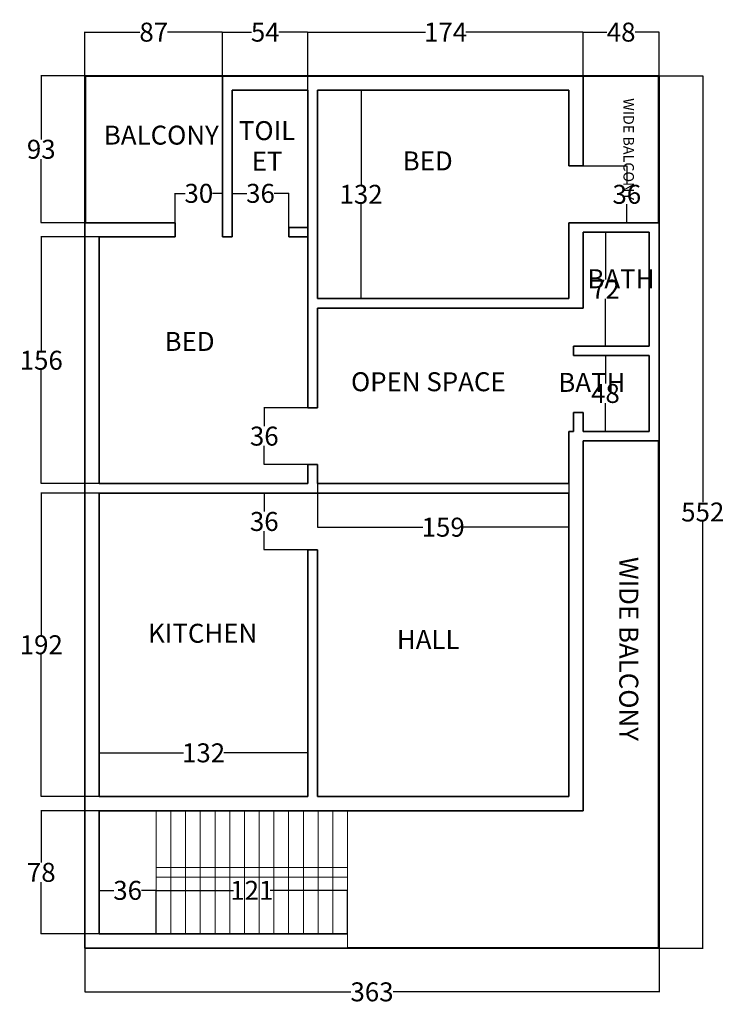
# Model space of a CAD drawing. Units: inches. Extents: x -24 to 1692, y -109 to 592.
# Tile 1 of 4: x -24 to 422, y -31 to 592. Entities that reach past the tile are written whole.
import ezdxf
from ezdxf.enums import TextEntityAlignment as Align

# ---------------------------------------------------------------- set-up
doc = ezdxf.new("R2010")
doc.units = ezdxf.units.IN
doc.header["$MEASUREMENT"] = 0
for name, color, linetype, lineweight in [('A-ANNO-DIMS', 2, 'Continuous', 18), ('A-AREA-IDEN', 7, 'Continuous', 18), ('A-FLOR-STRS', 2, 'Continuous', 18), ('A-WALL', 7, 'Continuous', 35)]:
    doc.layers.add(name, color=color, linetype=linetype, lineweight=lineweight)
doc.styles.get("Standard").update_dxf_attribs({"font": 'arial.ttf'})
doc.dimstyles.get("Standard").update_dxf_attribs({"dimtxt": 12, "dimasz": 0.18, "dimexe": 0.18, "dimexo": 0.0625, "dimgap": 0.09, "dimtad": 0, "dimtih": 1, "dimtoh": 1, "dimdec": 0, "dimzin": 0, "dimdsep": 46, "dimlunit": 4, "dimtxsty": 'Standard', "dimcen": 0.09, "dimadec": 0, "dimazin": 0, "dimtfac": 1, "dimtdec": 0, "dimtofl": 0, "dimtmove": 0, "dimatfit": 3, "dimfxl": 1, "dimtolj": 1, "dimtzin": 0, "dimarcsym": 0})

# ---------------------------------------------------------------- blocks, each defined once
blk = doc.blocks.new('*D11')
at = {"layer": 'A-ANNO-DIMS', "color": 0, "lineweight": -2, "transparency": 16777216}
for p, q in [((17.56, 4), (17.56, -23.73)), ((380.56, 4), (380.56, -23.73)), ((17.74, -23.55), (185.71, -23.55)), ((380.38, -23.55), (212.4, -23.55))]:
    blk.add_line(p, q, dxfattribs=at)
at = {"layer": 'A-ANNO-DIMS', "color": 0, "transparency": 16777216}
for points in [[(17.74, -23.52), (17.74, -23.58), (17.56, -23.55)], [(380.38, -23.52), (380.38, -23.58), (380.56, -23.55)]]:
    blk.add_solid(points, dxfattribs=at)
at = {"layer": 'Defpoints', "color": 0, "transparency": 16777216}
for p in [(17.56, 4.07), (380.56, 4.07), (380.56, -23.55)]:
    blk.add_point(p, dxfattribs=at)
at = {"layer": 'A-ANNO-DIMS', "color": 0, "transparency": 16777216, "insert": (199.06, -23.55), "char_height": 12, "attachment_point": 5}
blk.add_mtext('\\A1;363', dxfattribs=at)
blk = doc.blocks.new('*D12')
at = {"layer": 'A-ANNO-DIMS', "color": 0, "lineweight": -2, "transparency": 16777216}
for p, q in [((380.62, 556.07), (408.35, 556.07)), ((408.17, 555.89), (408.17, 286.28)), ((408.17, 4.25), (408.17, 273.85)), ((380.62, 4.07), (408.35, 4.07))]:
    blk.add_line(p, q, dxfattribs=at)
at = {"layer": 'A-ANNO-DIMS', "color": 0, "transparency": 16777216}
for points in [[(408.14, 555.89), (408.2, 555.89), (408.17, 556.07)], [(408.14, 4.25), (408.2, 4.25), (408.17, 4.07)]]:
    blk.add_solid(points, dxfattribs=at)
at = {"layer": 'Defpoints', "color": 0, "transparency": 16777216}
for p in [(380.56, 556.07), (408.17, 556.07), (380.56, 4.07)]:
    blk.add_point(p, dxfattribs=at)
at = {"layer": 'A-ANNO-DIMS', "color": 0, "transparency": 16777216, "insert": (408.17, 280.07), "char_height": 12, "attachment_point": 5}
blk.add_mtext('\\A1;552', dxfattribs=at)
blk = doc.blocks.new('*D13')
at = {"layer": 'A-ANNO-DIMS', "color": 0, "lineweight": -2, "transparency": 16777216}
for p, q in [((17.56, 556.13), (17.56, 583.86)), ((17.74, 583.68), (52.36, 583.68)), ((104.38, 583.68), (69.75, 583.68)), ((104.56, 555.83), (104.56, 583.86))]:
    blk.add_line(p, q, dxfattribs=at)
at = {"layer": 'A-ANNO-DIMS', "color": 0, "transparency": 16777216}
for points in [[(17.74, 583.71), (17.74, 583.65), (17.56, 583.68)], [(104.38, 583.71), (104.38, 583.65), (104.56, 583.68)]]:
    blk.add_solid(points, dxfattribs=at)
at = {"layer": 'Defpoints', "color": 0, "transparency": 16777216}
for p in [(104.56, 583.68), (17.56, 556.07), (104.56, 555.77)]:
    blk.add_point(p, dxfattribs=at)
at = {"layer": 'A-ANNO-DIMS', "color": 0, "transparency": 16777216, "insert": (61.06, 583.68), "char_height": 12, "attachment_point": 5}
blk.add_mtext('\\A1;87', dxfattribs=at)
blk = doc.blocks.new('*D14')
at = {"layer": 'A-ANNO-DIMS', "color": 0, "lineweight": -2, "transparency": 16777216}
for p, q in [((104.56, 555.83), (104.56, 583.86)), ((104.74, 583.68), (122.9, 583.68)), ((158.38, 583.68), (140.22, 583.68)), ((158.56, 547.13), (158.56, 583.86))]:
    blk.add_line(p, q, dxfattribs=at)
at = {"layer": 'A-ANNO-DIMS', "color": 0, "transparency": 16777216}
for points in [[(104.74, 583.71), (104.74, 583.65), (104.56, 583.68)], [(158.38, 583.71), (158.38, 583.65), (158.56, 583.68)]]:
    blk.add_solid(points, dxfattribs=at)
at = {"layer": 'Defpoints', "color": 0, "transparency": 16777216}
for p in [(158.56, 583.68), (104.56, 555.77), (158.56, 547.07)]:
    blk.add_point(p, dxfattribs=at)
at = {"layer": 'A-ANNO-DIMS', "color": 0, "transparency": 16777216, "insert": (131.56, 583.68), "char_height": 12, "attachment_point": 5}
blk.add_mtext('\\A1;54', dxfattribs=at)
blk = doc.blocks.new('*D15')
at = {"layer": 'A-ANNO-DIMS', "color": 0, "lineweight": -2, "transparency": 16777216}
for p, q in [((158.56, 547.13), (158.56, 583.86)), ((158.74, 583.68), (232.8, 583.68)), ((332.38, 583.68), (258.31, 583.68)), ((332.56, 556.13), (332.56, 583.86))]:
    blk.add_line(p, q, dxfattribs=at)
at = {"layer": 'A-ANNO-DIMS', "color": 0, "transparency": 16777216}
for points in [[(158.74, 583.71), (158.74, 583.65), (158.56, 583.68)], [(332.38, 583.71), (332.38, 583.65), (332.56, 583.68)]]:
    blk.add_solid(points, dxfattribs=at)
at = {"layer": 'Defpoints', "color": 0, "transparency": 16777216}
for p in [(332.56, 583.68), (332.56, 556.07), (158.56, 547.07)]:
    blk.add_point(p, dxfattribs=at)
at = {"layer": 'A-ANNO-DIMS', "color": 0, "transparency": 16777216, "insert": (245.56, 583.68), "char_height": 12, "attachment_point": 5}
blk.add_mtext('\\A1;174', dxfattribs=at)
blk = doc.blocks.new('*D16')
at = {"layer": 'A-ANNO-DIMS', "color": 0, "lineweight": -2, "transparency": 16777216}
for p, q in [((332.56, 556.13), (332.56, 583.86)), ((332.74, 583.68), (347.62, 583.68)), ((380.38, 583.68), (365.49, 583.68)), ((380.56, 556.13), (380.56, 583.86))]:
    blk.add_line(p, q, dxfattribs=at)
at = {"layer": 'A-ANNO-DIMS', "color": 0, "transparency": 16777216}
for points in [[(332.74, 583.71), (332.74, 583.65), (332.56, 583.68)], [(380.38, 583.71), (380.38, 583.65), (380.56, 583.68)]]:
    blk.add_solid(points, dxfattribs=at)
at = {"layer": 'Defpoints', "color": 0, "transparency": 16777216}
for p in [(380.56, 583.68), (332.56, 556.07), (380.56, 556.07)]:
    blk.add_point(p, dxfattribs=at)
at = {"layer": 'A-ANNO-DIMS', "color": 0, "transparency": 16777216, "insert": (356.56, 583.68), "char_height": 12, "attachment_point": 5}
blk.add_mtext('\\A1;48', dxfattribs=at)
blk = doc.blocks.new('*D17')
at = {"layer": 'A-ANNO-DIMS', "color": 0, "lineweight": -2, "transparency": 16777216}
for p, q in [((26.49, 91.07), (-10.24, 91.07)), ((-10.06, 90.89), (-10.06, 58.28)), ((-10.06, 13.25), (-10.06, 45.85)), ((26.49, 13.07), (-10.24, 13.07))]:
    blk.add_line(p, q, dxfattribs=at)
at = {"layer": 'A-ANNO-DIMS', "color": 0, "transparency": 16777216}
for points in [[(-10.09, 90.89), (-10.03, 90.89), (-10.06, 91.07)], [(-10.09, 13.25), (-10.03, 13.25), (-10.06, 13.07)]]:
    blk.add_solid(points, dxfattribs=at)
at = {"layer": 'Defpoints', "color": 0, "transparency": 16777216}
for p in [(-10.06, 91.07), (26.56, 91.07), (26.56, 13.07)]:
    blk.add_point(p, dxfattribs=at)
at = {"layer": 'A-ANNO-DIMS', "color": 0, "transparency": 16777216, "insert": (-10.06, 52.07), "char_height": 12, "attachment_point": 5}
blk.add_mtext('\\A1;78', dxfattribs=at)
blk = doc.blocks.new('*D18')
at = {"layer": 'A-ANNO-DIMS', "color": 0, "lineweight": -2, "transparency": 16777216}
for p, q in [((26.49, 292.07), (-10.24, 292.07)), ((-10.06, 291.89), (-10.06, 202.28)), ((-10.06, 100.25), (-10.06, 189.85)), ((26.49, 100.07), (-10.24, 100.07))]:
    blk.add_line(p, q, dxfattribs=at)
at = {"layer": 'A-ANNO-DIMS', "color": 0, "transparency": 16777216}
for points in [[(-10.09, 291.89), (-10.03, 291.89), (-10.06, 292.07)], [(-10.09, 100.25), (-10.03, 100.25), (-10.06, 100.07)]]:
    blk.add_solid(points, dxfattribs=at)
at = {"layer": 'Defpoints', "color": 0, "transparency": 16777216}
for p in [(-10.06, 292.07), (26.56, 292.07), (26.56, 100.07)]:
    blk.add_point(p, dxfattribs=at)
at = {"layer": 'A-ANNO-DIMS', "color": 0, "transparency": 16777216, "insert": (-10.06, 196.07), "char_height": 12, "attachment_point": 5}
blk.add_mtext('\\A1;192', dxfattribs=at)
blk = doc.blocks.new('*D19')
at = {"layer": 'A-ANNO-DIMS', "color": 0, "lineweight": -2, "transparency": 16777216}
for p, q in [((26.49, 454.07), (-10.24, 454.07)), ((-10.06, 453.89), (-10.06, 382.28)), ((-10.06, 298.25), (-10.06, 369.85)), ((26.49, 298.07), (-10.24, 298.07))]:
    blk.add_line(p, q, dxfattribs=at)
at = {"layer": 'A-ANNO-DIMS', "color": 0, "transparency": 16777216}
for points in [[(-10.09, 453.89), (-10.03, 453.89), (-10.06, 454.07)], [(-10.09, 298.25), (-10.03, 298.25), (-10.06, 298.07)]]:
    blk.add_solid(points, dxfattribs=at)
at = {"layer": 'Defpoints', "color": 0, "transparency": 16777216}
for p in [(-10.06, 454.07), (26.56, 454.07), (26.56, 298.07)]:
    blk.add_point(p, dxfattribs=at)
at = {"layer": 'A-ANNO-DIMS', "color": 0, "transparency": 16777216, "insert": (-10.06, 376.07), "char_height": 12, "attachment_point": 5}
blk.add_mtext('\\A1;156', dxfattribs=at)
blk = doc.blocks.new('*D20')
at = {"layer": 'A-ANNO-DIMS', "color": 0, "lineweight": -2, "transparency": 16777216}
for p, q in [((17.49, 556.07), (-10.24, 556.07)), ((-10.06, 555.89), (-10.06, 515.79)), ((-10.06, 463.25), (-10.06, 503.34)), ((17.49, 463.07), (-10.24, 463.07))]:
    blk.add_line(p, q, dxfattribs=at)
at = {"layer": 'A-ANNO-DIMS', "color": 0, "transparency": 16777216}
for points in [[(-10.09, 555.89), (-10.03, 555.89), (-10.06, 556.07)], [(-10.09, 463.25), (-10.03, 463.25), (-10.06, 463.07)]]:
    blk.add_solid(points, dxfattribs=at)
at = {"layer": 'Defpoints', "color": 0, "transparency": 16777216}
for p in [(-10.06, 556.07), (17.56, 556.07), (17.56, 463.07)]:
    blk.add_point(p, dxfattribs=at)
at = {"layer": 'A-ANNO-DIMS', "color": 0, "transparency": 16777216, "insert": (-10.06, 509.57), "char_height": 12, "attachment_point": 5}
blk.add_mtext('\\A1;93', dxfattribs=at)
blk = doc.blocks.new('*D21')
at = {"layer": 'A-ANNO-DIMS', "color": 0, "lineweight": -2, "transparency": 16777216}
for p, q in [((164.62, 547.07), (192.35, 547.07)), ((192.17, 546.89), (192.17, 487.29)), ((192.17, 415.25), (192.17, 474.84)), ((164.62, 415.07), (192.35, 415.07))]:
    blk.add_line(p, q, dxfattribs=at)
at = {"layer": 'A-ANNO-DIMS', "color": 0, "transparency": 16777216}
for points in [[(192.14, 546.89), (192.2, 546.89), (192.17, 547.07)], [(192.14, 415.25), (192.2, 415.25), (192.17, 415.07)]]:
    blk.add_solid(points, dxfattribs=at)
at = {"layer": 'Defpoints', "color": 0, "transparency": 16777216}
for p in [(164.56, 547.07), (164.56, 415.07), (192.17, 415.07)]:
    blk.add_point(p, dxfattribs=at)
at = {"layer": 'A-ANNO-DIMS', "color": 0, "transparency": 16777216, "insert": (192.17, 481.07), "char_height": 12, "attachment_point": 5}
blk.add_mtext('\\A1;132', dxfattribs=at)
blk = doc.blocks.new('*D22')
at = {"layer": 'A-ANNO-DIMS', "color": 0, "lineweight": -2, "transparency": 16777216}
for p, q in [((374.19, 457.07), (346.46, 457.07)), ((346.64, 456.89), (346.64, 427.18)), ((346.64, 385.25), (346.64, 414.95)), ((374.19, 385.07), (346.46, 385.07))]:
    blk.add_line(p, q, dxfattribs=at)
at = {"layer": 'A-ANNO-DIMS', "color": 0, "transparency": 16777216}
for points in [[(346.61, 456.89), (346.67, 456.89), (346.64, 457.07)], [(346.61, 385.25), (346.67, 385.25), (346.64, 385.07)]]:
    blk.add_solid(points, dxfattribs=at)
at = {"layer": 'Defpoints', "color": 0, "transparency": 16777216}
for p in [(346.64, 457.07), (374.26, 457.07), (374.26, 385.07)]:
    blk.add_point(p, dxfattribs=at)
at = {"layer": 'A-ANNO-DIMS', "color": 0, "transparency": 16777216, "insert": (346.64, 421.07), "char_height": 12, "attachment_point": 5}
blk.add_mtext('\\A1;72', dxfattribs=at)
blk = doc.blocks.new('*D23')
at = {"layer": 'A-ANNO-DIMS', "color": 0, "lineweight": -2, "transparency": 16777216}
for p, q in [((374.19, 379.07), (346.46, 379.07)), ((346.64, 378.89), (346.64, 361.28)), ((346.64, 331.25), (346.64, 348.85)), ((374.19, 331.07), (346.46, 331.07))]:
    blk.add_line(p, q, dxfattribs=at)
at = {"layer": 'A-ANNO-DIMS', "color": 0, "transparency": 16777216}
for points in [[(346.61, 378.89), (346.67, 378.89), (346.64, 379.07)], [(346.61, 331.25), (346.67, 331.25), (346.64, 331.07)]]:
    blk.add_solid(points, dxfattribs=at)
at = {"layer": 'Defpoints', "color": 0, "transparency": 16777216}
for p in [(346.64, 379.07), (374.26, 379.07), (374.26, 331.07)]:
    blk.add_point(p, dxfattribs=at)
at = {"layer": 'A-ANNO-DIMS', "color": 0, "transparency": 16777216, "insert": (346.64, 355.07), "char_height": 12, "attachment_point": 5}
blk.add_mtext('\\A1;48', dxfattribs=at)
blk = doc.blocks.new('*D24')
at = {"layer": 'A-ANNO-DIMS', "color": 0, "lineweight": -2, "transparency": 16777216}
for p, q in [((26.56, 13.13), (26.56, 40.86)), ((26.74, 40.68), (35.88, 40.68)), ((62.38, 40.68), (53.23, 40.68)), ((62.56, 13.13), (62.56, 40.86))]:
    blk.add_line(p, q, dxfattribs=at)
at = {"layer": 'A-ANNO-DIMS', "color": 0, "transparency": 16777216}
for points in [[(26.74, 40.71), (26.74, 40.65), (26.56, 40.68)], [(62.38, 40.71), (62.38, 40.65), (62.56, 40.68)]]:
    blk.add_solid(points, dxfattribs=at)
at = {"layer": 'Defpoints', "color": 0, "transparency": 16777216}
for p in [(62.56, 40.68), (26.56, 13.07), (62.56, 13.07)]:
    blk.add_point(p, dxfattribs=at)
at = {"layer": 'A-ANNO-DIMS', "color": 0, "transparency": 16777216, "insert": (44.56, 40.68), "char_height": 12, "attachment_point": 5}
blk.add_mtext('\\A1;36', dxfattribs=at)
blk = doc.blocks.new('*D25')
at = {"layer": 'A-ANNO-DIMS', "color": 0, "lineweight": -2, "transparency": 16777216}
for p, q in [((62.56, 13.13), (62.56, 40.86)), ((62.74, 40.68), (111.43, 40.68)), ((183.38, 40.68), (134.68, 40.68)), ((183.56, 13.13), (183.56, 40.86))]:
    blk.add_line(p, q, dxfattribs=at)
at = {"layer": 'A-ANNO-DIMS', "color": 0, "transparency": 16777216}
for points in [[(62.74, 40.71), (62.74, 40.65), (62.56, 40.68)], [(183.38, 40.71), (183.38, 40.65), (183.56, 40.68)]]:
    blk.add_solid(points, dxfattribs=at)
at = {"layer": 'Defpoints', "color": 0, "transparency": 16777216}
for p in [(183.56, 40.68), (62.56, 13.07), (183.56, 13.07)]:
    blk.add_point(p, dxfattribs=at)
at = {"layer": 'A-ANNO-DIMS', "color": 0, "transparency": 16777216, "insert": (123.06, 40.68), "char_height": 12, "attachment_point": 5}
blk.add_mtext('\\A1;121', dxfattribs=at)
blk = doc.blocks.new('*D26')
at = {"layer": 'A-ANNO-DIMS', "color": 0, "lineweight": -2, "transparency": 16777216}
for p, q in [((26.56, 100.13), (26.56, 127.86)), ((26.74, 127.68), (79.84, 127.68)), ((158.38, 127.68), (105.28, 127.68)), ((158.56, 100.13), (158.56, 127.86))]:
    blk.add_line(p, q, dxfattribs=at)
at = {"layer": 'A-ANNO-DIMS', "color": 0, "transparency": 16777216}
for points in [[(26.74, 127.71), (26.74, 127.65), (26.56, 127.68)], [(158.38, 127.71), (158.38, 127.65), (158.56, 127.68)]]:
    blk.add_solid(points, dxfattribs=at)
at = {"layer": 'Defpoints', "color": 0, "transparency": 16777216}
for p in [(158.56, 127.68), (26.56, 100.07), (158.56, 100.07)]:
    blk.add_point(p, dxfattribs=at)
at = {"layer": 'A-ANNO-DIMS', "color": 0, "transparency": 16777216, "insert": (92.56, 127.68), "char_height": 12, "attachment_point": 5}
blk.add_mtext('\\A1;132', dxfattribs=at)
blk = doc.blocks.new('*D27')
at = {"layer": 'A-ANNO-DIMS', "color": 0, "lineweight": -2, "transparency": 16777216}
for p, q in [((74.56, 454.13), (74.56, 481.86)), ((74.74, 481.68), (80.9, 481.68)), ((104.38, 481.68), (98.22, 481.68)), ((104.56, 454.13), (104.56, 481.86))]:
    blk.add_line(p, q, dxfattribs=at)
at = {"layer": 'A-ANNO-DIMS', "color": 0, "transparency": 16777216}
for points in [[(74.74, 481.71), (74.74, 481.65), (74.56, 481.68)], [(104.38, 481.71), (104.38, 481.65), (104.56, 481.68)]]:
    blk.add_solid(points, dxfattribs=at)
at = {"layer": 'Defpoints', "color": 0, "transparency": 16777216}
for p in [(104.56, 481.68), (74.56, 454.07), (104.56, 454.07)]:
    blk.add_point(p, dxfattribs=at)
at = {"layer": 'A-ANNO-DIMS', "color": 0, "transparency": 16777216, "insert": (89.56, 481.68), "char_height": 12, "attachment_point": 5}
blk.add_mtext('\\A1;30', dxfattribs=at)
blk = doc.blocks.new('*D28')
at = {"layer": 'A-ANNO-DIMS', "color": 0, "lineweight": -2, "transparency": 16777216}
for p, q in [((110.56, 454.13), (110.56, 481.86)), ((110.74, 481.68), (119.88, 481.68)), ((146.38, 481.68), (137.23, 481.68)), ((146.56, 454.13), (146.56, 481.86))]:
    blk.add_line(p, q, dxfattribs=at)
at = {"layer": 'A-ANNO-DIMS', "color": 0, "transparency": 16777216}
for points in [[(110.74, 481.71), (110.74, 481.65), (110.56, 481.68)], [(146.38, 481.71), (146.38, 481.65), (146.56, 481.68)]]:
    blk.add_solid(points, dxfattribs=at)
at = {"layer": 'Defpoints', "color": 0, "transparency": 16777216}
for p in [(146.56, 481.68), (110.56, 454.07), (146.56, 454.07)]:
    blk.add_point(p, dxfattribs=at)
at = {"layer": 'A-ANNO-DIMS', "color": 0, "transparency": 16777216, "insert": (128.56, 481.68), "char_height": 12, "attachment_point": 5}
blk.add_mtext('\\A1;36', dxfattribs=at)
blk = doc.blocks.new('*D29')
at = {"layer": 'A-ANNO-DIMS', "color": 0, "lineweight": -2, "transparency": 16777216}
for p, q in [((332.62, 499.07), (360.35, 499.07)), ((360.17, 498.89), (360.17, 487.29)), ((360.17, 463.25), (360.17, 474.84)), ((332.62, 463.07), (360.35, 463.07))]:
    blk.add_line(p, q, dxfattribs=at)
at = {"layer": 'A-ANNO-DIMS', "color": 0, "transparency": 16777216}
for points in [[(360.14, 498.89), (360.2, 498.89), (360.17, 499.07)], [(360.14, 463.25), (360.2, 463.25), (360.17, 463.07)]]:
    blk.add_solid(points, dxfattribs=at)
at = {"layer": 'Defpoints', "color": 0, "transparency": 16777216}
for p in [(332.56, 499.07), (332.56, 463.07), (360.17, 463.07)]:
    blk.add_point(p, dxfattribs=at)
at = {"layer": 'A-ANNO-DIMS', "color": 0, "transparency": 16777216, "insert": (360.17, 481.07), "char_height": 12, "attachment_point": 5}
blk.add_mtext('\\A1;36', dxfattribs=at)
blk = doc.blocks.new('*D30')
at = {"layer": 'A-ANNO-DIMS', "color": 0, "lineweight": -2, "transparency": 16777216}
for p, q in [((158.49, 346.07), (130.76, 346.07)), ((130.94, 345.89), (130.94, 334.29)), ((130.94, 310.25), (130.94, 321.84)), ((158.49, 310.07), (130.76, 310.07))]:
    blk.add_line(p, q, dxfattribs=at)
at = {"layer": 'A-ANNO-DIMS', "color": 0, "transparency": 16777216}
for points in [[(130.91, 345.89), (130.97, 345.89), (130.94, 346.07)], [(130.91, 310.25), (130.97, 310.25), (130.94, 310.07)]]:
    blk.add_solid(points, dxfattribs=at)
at = {"layer": 'Defpoints', "color": 0, "transparency": 16777216}
for p in [(130.94, 346.07), (158.56, 346.07), (158.56, 310.07)]:
    blk.add_point(p, dxfattribs=at)
at = {"layer": 'A-ANNO-DIMS', "color": 0, "transparency": 16777216, "insert": (130.94, 328.07), "char_height": 12, "attachment_point": 5}
blk.add_mtext('\\A1;36', dxfattribs=at)
blk = doc.blocks.new('*D31')
at = {"layer": 'A-ANNO-DIMS', "color": 0, "lineweight": -2, "transparency": 16777216}
for p, q in [((158.49, 292.07), (130.76, 292.07)), ((130.94, 291.89), (130.94, 280.29)), ((130.94, 256.25), (130.94, 267.84)), ((158.49, 256.07), (130.76, 256.07))]:
    blk.add_line(p, q, dxfattribs=at)
at = {"layer": 'A-ANNO-DIMS', "color": 0, "transparency": 16777216}
for points in [[(130.91, 291.89), (130.97, 291.89), (130.94, 292.07)], [(130.91, 256.25), (130.97, 256.25), (130.94, 256.07)]]:
    blk.add_solid(points, dxfattribs=at)
at = {"layer": 'Defpoints', "color": 0, "transparency": 16777216}
for p in [(130.94, 292.07), (158.56, 292.07), (158.56, 256.07)]:
    blk.add_point(p, dxfattribs=at)
at = {"layer": 'A-ANNO-DIMS', "color": 0, "transparency": 16777216, "insert": (130.94, 274.07), "char_height": 12, "attachment_point": 5}
blk.add_mtext('\\A1;36', dxfattribs=at)
blk = doc.blocks.new('*D32')
at = {"layer": 'A-ANNO-DIMS', "color": 0, "lineweight": -2, "transparency": 16777216}
for p, q in [((164.56, 298), (164.56, 270.27)), ((323.56, 298), (323.56, 270.27)), ((164.74, 270.45), (231.26, 270.45)), ((323.38, 270.45), (256.85, 270.45))]:
    blk.add_line(p, q, dxfattribs=at)
at = {"layer": 'A-ANNO-DIMS', "color": 0, "transparency": 16777216}
for points in [[(164.74, 270.48), (164.74, 270.42), (164.56, 270.45)], [(323.38, 270.48), (323.38, 270.42), (323.56, 270.45)]]:
    blk.add_solid(points, dxfattribs=at)
at = {"layer": 'Defpoints', "color": 0, "transparency": 16777216}
for p in [(164.56, 298.07), (323.56, 298.07), (164.56, 270.45)]:
    blk.add_point(p, dxfattribs=at)
at = {"layer": 'A-ANNO-DIMS', "color": 0, "transparency": 16777216, "insert": (244.06, 270.45), "char_height": 12, "attachment_point": 5}
blk.add_mtext('\\A1;159', dxfattribs=at)

msp = doc.modelspace()

# ---------------------------------------------------------------- linework, layer by layer
at = {"layer": 'A-FLOR-STRS'}
for p, q in [((26.5561, 91.0656), (183.5561, 91.0656)), ((26.5561, 13.0656), (26.5561, 91.0656)), ((62.5561, 13.0656), (62.5561, 91.0656)), ((71.8661, 13.0656), (71.8661, 91.0656)), ((81.1761, 13.0656), (81.1761, 91.0656)), ((90.4861, 13.0656), (90.4861, 91.0656)), ((99.7961, 13.0656), (99.7961, 91.0656)), ((109.1061, 13.0656), (109.1061, 91.0656)), ((118.4161, 13.0656), (118.4161, 91.0656)), ((127.7261, 13.0656), (127.7261, 91.0656)), ((137.0361, 13.0656), (137.0361, 91.0656)), ((146.3461, 13.0656), (146.3461, 91.0656)), ((155.6561, 13.0656), (155.6561, 91.0656)), ((164.9661, 13.0656), (164.9661, 91.0656)), ((174.2761, 13.0656), (174.2761, 91.0656)), ((183.5561, 91.0656), (183.5561, 4.0656)), ((62.5561, 55.0656), (183.5561, 55.0656)), ((183.5561, 49.0656), (62.5561, 49.0656)), ((183.5561, 13.0656), (26.5561, 13.0656))]:
    msp.add_line(p, q, dxfattribs=at)
at = {"layer": 'A-WALL'}
for p, q in [((380.5561, 556.0656), (17.5561, 556.0656)), ((17.5561, 556.0656), (17.5561, 4.0656)), ((101.5561, 555.7656), (17.5561, 555.7656)), ((380.5561, 555.7656), (17.5561, 555.7656)), ((17.8561, 556.0656), (17.8561, 463.0656)), ((104.5561, 555.7656), (104.5561, 463.0656)), ((332.5561, 556.0656), (332.5561, 499.0656)), ((380.2561, 463.0656), (380.2561, 556.0656)), ((380.5561, 4.0656), (380.5561, 556.0656)), ((110.5561, 547.0656), (110.5561, 463.0656)), ((158.5561, 547.0656), (110.5561, 547.0656)), ((158.5561, 547.0656), (158.5561, 454.0656)), ((323.5561, 547.0656), (164.5561, 547.0656)), ((164.5561, 547.0656), (164.5561, 415.0656)), ((323.5561, 547.0656), (323.5561, 499.0656)), ((332.5561, 499.0656), (323.5561, 499.0656)), ((74.5561, 463.0656), (17.5561, 463.0656)), ((74.5561, 463.0656), (74.5561, 454.0656)), ((74.5561, 463.0656), (74.5561, 454.0656)), ((104.5561, 463.0656), (104.5561, 454.0656)), ((110.5561, 463.0656), (110.5561, 454.0656)), ((332.5561, 463.0656), (323.5561, 463.0656)), ((323.5561, 463.0656), (323.5561, 415.0656)), ((380.5561, 463.0656), (332.5561, 463.0656)), ((158.5561, 460.0656), (146.5561, 460.0656)), ((146.5561, 460.0656), (146.5561, 454.0656)), ((158.5561, 457.0656), (158.5561, 346.0656)), ((332.5561, 457.0656), (332.5561, 409.0656)), ((374.2561, 457.0656), (332.5561, 457.0656)), ((374.2561, 385.0656), (374.2561, 457.0656)), ((26.5561, 454.0656), (26.5561, 298.0656)), ((74.5561, 454.0656), (26.5561, 454.0656)), ((110.5561, 454.0656), (104.5561, 454.0656)), ((158.5561, 454.0656), (146.5561, 454.0656)), ((323.5561, 415.0656), (164.5561, 415.0656)), ((164.5561, 409.0656), (164.5561, 346.0656)), ((332.5561, 409.0656), (164.5561, 409.0656)), ((374.2561, 385.0656), (326.5561, 385.0656)), ((326.5561, 385.0656), (326.5561, 379.0656)), ((380.5561, 385.0656), (380.2561, 385.0656)), ((374.2561, 379.0656), (326.5561, 379.0656)), ((374.2561, 331.0656), (374.2561, 379.0656)), ((380.5561, 379.0656), (380.2561, 379.0656)), ((158.5561, 346.0656), (164.5561, 346.0656)), ((326.5561, 343.0656), (326.5561, 331.0656)), ((332.5561, 343.0656), (326.5561, 343.0656)), ((332.5561, 343.0656), (332.5561, 331.0656)), ((323.5561, 331.0656), (323.5561, 298.0656)), ((326.5561, 331.0656), (323.5561, 331.0656)), ((374.2561, 331.0656), (332.5561, 331.0656)), ((380.2561, 325.0656), (332.5561, 325.0656)), ((332.5561, 325.0656), (332.5561, 91.0656)), ((380.2561, 4.3656), (380.2561, 325.0656)), ((158.5561, 310.0656), (164.5561, 310.0656)), ((158.5561, 310.0656), (158.5561, 298.0656)), ((164.5561, 310.0656), (164.5561, 298.0656)), ((158.5561, 298.0656), (26.5561, 298.0656)), ((323.5561, 298.0656), (164.5561, 298.0656)), ((26.5561, 292.0656), (26.5561, 100.0656)), ((158.5561, 292.0656), (26.5561, 292.0656)), ((158.5561, 292.0656), (164.5561, 292.0656)), ((323.5561, 292.0656), (164.5561, 292.0656)), ((323.5561, 292.0656), (323.5561, 100.0656)), ((158.5561, 256.0656), (158.5561, 100.0656)), ((158.5561, 256.0656), (164.5561, 256.0656)), ((164.5561, 256.0656), (164.5561, 100.0656)), ((158.5561, 100.0656), (26.5561, 100.0656)), ((323.5561, 100.0656), (164.5561, 100.0656)), ((332.5561, 91.0656), (26.5561, 91.0656)), ((26.5561, 91.0656), (26.5561, 13.0656)), ((26.5561, 13.0656), (183.5561, 13.0656)), ((17.5561, 4.0656), (380.5561, 4.0656)), ((183.5561, 4.3656), (380.2561, 4.3656))]:
    msp.add_line(p, q, dxfattribs=at)

# ---------------------------------------------------------------- texts
at = {"layer": 'A-AREA-IDEN'}
for height, p in [(6.63899, (358.0324, 509.6639)), (12, (355.4218, 193.4544))]:
    msp.add_text('WIDE BALCONY', height=height, rotation=270, dxfattribs=at).set_placement(p, align=Align.CENTER)
for s, p in [('BALCONY', (65.8539, 512.5114)), ('TOIL', (132.7037, 515.3591)), ('ET', (132.7037, 496.0821)), ('BED', (234.2739, 496.202)), ('BATH', (356.436, 421.6402)), ('BED', (83.726, 381.9812)), ('OPEN SPACE', (234.688, 356.4727)), ('BATH', (338.0697, 356.0726)), ('KITCHEN', (91.9988, 197.3289)), ('HALL', (234.5995, 193.4255))]:
    msp.add_text(s, height=12, dxfattribs=at).set_placement(p, align=Align.CENTER)

# ---------------------------------------------------------------- dimensions: what is measured, and where the dimension line sits
at = {"layer": 'A-ANNO-DIMS'}
for base, p1, p2, picture, middle in [((104.5561, 583.6806), (17.5561, 556.0656), (104.5561, 555.7656), '*D13', (61.0561, 583.6806)), ((158.5561, 583.6806), (104.5561, 555.7656), (158.5561, 547.0656), '*D14', (131.5561, 583.6806)), ((332.5561, 583.6806), (158.5561, 547.0656), (332.5561, 556.0656), '*D15', (245.5561, 583.6806)), ((380.5561, 583.6806), (332.5561, 556.0656), (380.5561, 556.0656), '*D16', (356.5561, 583.6806)), ((104.5561, 481.6806), (74.5561, 454.0656), (104.5561, 454.0656), '*D27', (89.5561, 481.6806)), ((146.5561, 481.6806), (110.5561, 454.0656), (146.5561, 454.0656), '*D28', (128.5561, 481.6806)), ((158.5561, 127.6806), (26.5561, 100.0656), (158.5561, 100.0656), '*D26', (92.5561, 127.6806)), ((62.5561, 40.6806), (26.5561, 13.0656), (62.5561, 13.0656), '*D24', (44.5561, 40.6806)), ((183.5561, 40.6806), (62.5561, 13.0656), (183.5561, 13.0656), '*D25', (123.0561, 40.6806)), ((380.5561, -23.5494), (17.5561, 4.0656), (380.5561, 4.0656), '*D11', (199.0561, -23.5494))]:
    dim = msp.add_linear_dim(base=base, p1=p1, p2=p2, dimstyle='Standard', override={"dimdec": 0, "dimlfac": 1, "dimrnd": 0, "dimzin": 0, "dimdsep": 46, "dimlunit": 2}, dxfattribs=at)
    dim.commit()
    dim.dimension.update_dxf_attribs({"geometry": picture, "text_midpoint": middle})
for base, p1, p2, angle, picture, middle in [((-10.0589, 556.0656), (17.5561, 463.0656), (17.5561, 556.0656), 90, '*D20', (-10.0589, 509.5656)), ((408.1711, 556.0656), (380.5561, 4.0656), (380.5561, 556.0656), 90, '*D12', (408.1711, 280.0656)), ((192.1711, 415.0656), (164.5561, 547.0656), (164.5561, 415.0656), 270, '*D21', (192.1711, 481.0656)), ((360.1711, 463.0656), (332.5561, 499.0656), (332.5561, 463.0656), 270, '*D29', (360.1711, 481.0656)), ((346.6411, 457.0656), (374.2561, 385.0656), (374.2561, 457.0656), 90, '*D22', (346.6411, 421.0656)), ((-10.0589, 454.0656), (26.5561, 298.0656), (26.5561, 454.0656), 90, '*D19', (-10.0589, 376.0656)), ((346.6411, 379.0656), (374.2561, 331.0656), (374.2561, 379.0656), 90, '*D23', (346.6411, 355.0656)), ((130.9411, 346.0656), (158.5561, 310.0656), (158.5561, 346.0656), 90, '*D30', (130.9411, 328.0656)), ((164.5561, 270.4506), (323.5561, 298.0656), (164.5561, 298.0656), 180, '*D32', (244.0561, 270.4506)), ((-10.0589, 292.0656), (26.5561, 100.0656), (26.5561, 292.0656), 90, '*D18', (-10.0589, 196.0656)), ((130.9411, 292.0656), (158.5561, 256.0656), (158.5561, 292.0656), 90, '*D31', (130.9411, 274.0656)), ((-10.0589, 91.0656), (26.5561, 13.0656), (26.5561, 91.0656), 90, '*D17', (-10.0589, 52.0656))]:
    dim = msp.add_linear_dim(base=base, p1=p1, p2=p2, angle=angle, dimstyle='Standard', override={"dimdec": 0, "dimlfac": 1, "dimrnd": 0, "dimzin": 0, "dimdsep": 46, "dimlunit": 2}, dxfattribs=at)
    dim.commit()
    dim.dimension.update_dxf_attribs({"geometry": picture, "text_midpoint": middle})

doc.saveas('drawing.dxf')
